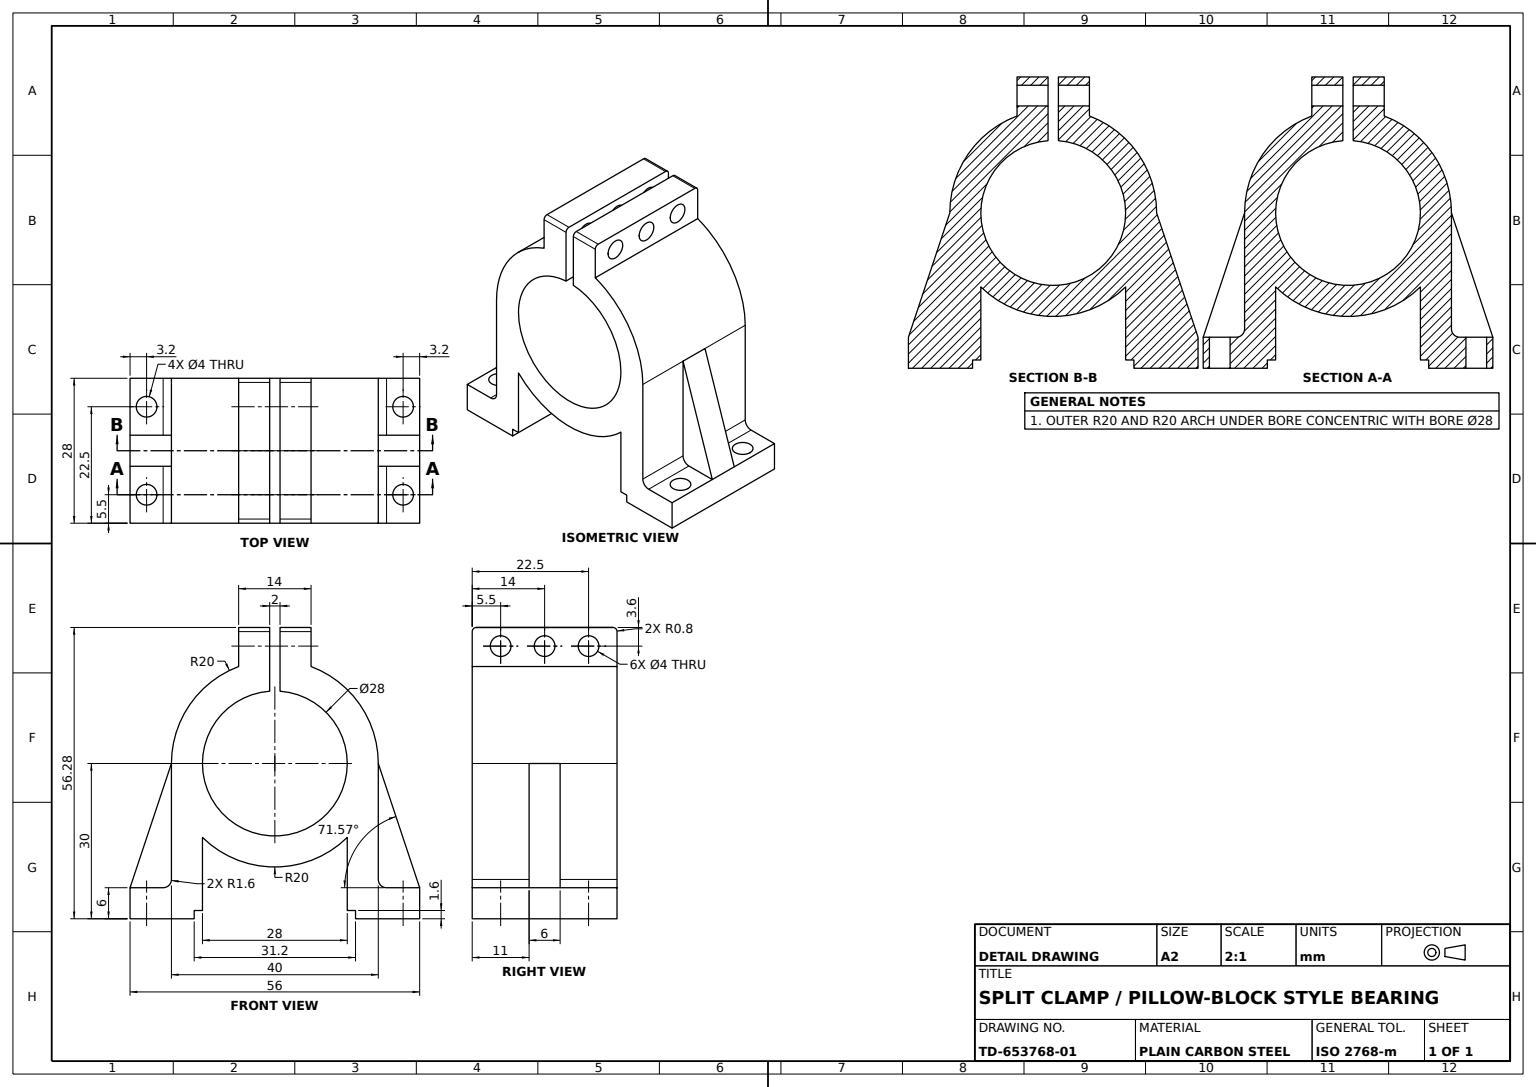
SolidWorks part; units mm, degrees
material "Plain Carbon Steel"
ref_plane "Front Plane" through (0, 0, 0) normal (0, 0, 1) x (1, 0, 0)
ref_plane "Top Plane" through (0, 0, 0) normal (0, 1, 0) x (1, 0, 0)
ref_plane "Right Plane" through (0, 0, 0) normal (1, 0, 0) x (0, 0, -1)
sketch "Clamp Body Profile" plane through (0, 0, 0) normal (0, 0, 1) x (1, 0, 0)
  line L6 (0, 0) -> (0, 4)
  line L7 (20, 24) -> (20, 0)
  line L8 (20, 0) -> (28, 0)
  line L9 (28, 0) -> (28, -6)
  line L16 (28, -6) -> (15.6, -6)
  line L17 (15.6, -6) -> (15.6, -4.4)
  line L18 (15.6, -4.4) -> (14, -4.4)
  line L19 (14, -4.4) -> (14, 9.7171)
  line L20 (-20, 24) -> (-20, 0)
  line L21 (-20, 0) -> (-28, 0)
  line L22 (-28, 0) -> (-28, -6)
  line L23 (-28, -6) -> (-15.6, -6)
  line L24 (-15.6, -6) -> (-15.6, -4.4)
  line L25 (-15.6, -4.4) -> (-14, -4.4)
  line L26 (-14, -4.4) -> (-14, 9.7171)
  arc A1 (-14, 9.7171) -> (14, 9.7171) centre (0, 24) ccw
  arc A2 (20, 24) -> (-20, 24) centre (0, 24) ccw
  dimension "D1" = 14
  dimension "D3" = 40
  dimension "D4" = 24
  dimension "D13" = 24
  dimension "D2" = 14
  dimension "D5" = 28
  dimension "D6" = 6
  dimension "D7" = 1.6
  dimension "D8" = 1.6
  dimension "D9" = 14.1171
  dimension "D10" = 6
  dimension "D11" = 1.6
  dimension "D12" = 6
extrude "Clamp Body" add sketch "Clamp Body Profile" along normal mid plane 28 contours L7 A2 L20 L21 L22 L23 L24 L25 L26 A1 L19 L18 L17 L16 L9 L8
sketch "Clamp Bore Sketch" plane through (0, 0, 14) normal (0, 0, 1) x (1, 0, 0)
  circle A0 centre (0, 24) radius 14
  dimension "D1" = 28
extrude "Clamp Bore" cut sketch "Clamp Bore Sketch" against normal blind 96
sketch "Clamp Lugs Sketch" plane through (0, 0, 14) normal (0, 0, 1) x (1, 0, 0)
  line L0 (0, 38) -> (7, 38)
  line L1 (7, 38) -> (7, 42.735)
  line L2 (7, 42.735) -> (7, 50.2788)
  line L3 (7, 50.2788) -> (-7, 50.2788)
  line L4 (-7, 50.2788) -> (-7, 38)
  line L5 (-7, 38) -> (0, 38)
  line L6 (-28, 0) -> (-28, -6) construction
  line L7 (-28, -6) -> (-15.6, -6) construction
  circle A0 centre (0, 24) radius 14 construction
  arc A1 (20, 24) -> (-20, 24) centre (0, 24) ccw construction
  dimension "D1" = 21
  dimension "D2" = 28
  dimension "D3" = 56.2788
extrude "Clamp Lugs" add sketch "Clamp Lugs Sketch" against normal blind 28
sketch "Split Slot Sketch" plane through (0, 0, 14) normal (0, 0, 1) x (1, 0, 0)
  line L0 (-1, 37.9642) -> (-1, 37.4063)
  line L1 (1, 38) -> (1, 50.2788)
  line L2 (7, 50.2788) -> (-7, 50.2788) construction
  line L3 (1, 50.2788) -> (-1, 50.2788)
  line L4 (-1, 50.2788) -> (-1, 37.9642)
  line L5 (-1, 37.4063) -> (1, 37.4063)
  line L6 (1, 37.4063) -> (1, 38)
  circle A0 centre (0, 24) radius 14 construction
  dimension "D1" = 2
  dimension "D2" = 12.2788
  dimension "D3" = 12.3145
  dimension "D4" = 12.8725
extrude "Split Slot 2mm" cut sketch "Split Slot Sketch" against normal blind 52
fillet "Body Fillet R1.6 A" radius 1.6 1 edges at (20, 0, 0)
fillet "Body Fillet R1.6 B" radius 1.6 1 edges at (-20, 0, 0)
sketch "Clamp Screw Holes Sketch" plane through (7, 0, 0) normal (1, 0, 0) x (0, 0, -1)
  line L0 (14, 42.735) -> (14, 50.2788) construction
  line L1 (14, 42.735) -> (-14, 42.735) construction
  circle A0 centre (8.5, 46.6788) radius 2
  circle A1 centre (-8.5, 46.6788) radius 2
  circle A2 centre (0, 46.6788) radius 2
  dimension "D1" = 4
  dimension "D2" = 5.5
  dimension "D3" = 14
  dimension "D4" = 22.5
  dimension "D5" = 3.9438
extrude "Clamp Screw Holes 3x" cut sketch "Clamp Screw Holes Sketch" against normal blind 52
sketch "Support Rib 1 Sketch" plane through (0, 0, 0) normal (0, 0, 1) x (1, 0, 0)
  line L0 (28, 0) -> (20, 24)
rib "Support Rib 1" sketch "Support Rib 1 Sketch" sketch "Support Rib 1 Sketch" thickness 6 extrusion direction parallel to sketch draft on no parameters "D1"=6
sketch "Support Rib 2 Sketch" plane through (0, 0, 0) normal (0, 0, 1) x (1, 0, 0)
  line L0 (-20, 24) -> (-28, 0)
rib "Support Rib 2" sketch "Support Rib 2 Sketch" sketch "Support Rib 2 Sketch" thickness 6 extrusion direction parallel to sketch draft on no parameters "D1"=6
sketch "Base Mounting Holes Sketch" plane through (0, 0, 0) normal (0, 1, 0) x (1, 0, 0)
  line L0 (21.6, -3) -> (21.6, -14) construction
  line L1 (21.6, -3) -> (28, -3) construction
  circle A0 centre (24.8, 8.5) radius 2
  circle A1 centre (24.8, -8.5) radius 2
  circle A2 centre (-24.8, 8.5) radius 2
  circle A3 centre (-24.8, -8.5) radius 2
  dimension "D1" = 4
  dimension "D2" = 3.2
  dimension "D3" = 46.4
  dimension "D4" = 11.5
  dimension "D5" = 5.5
extrude "Base Mounting Holes 4x" cut sketch "Base Mounting Holes Sketch" against normal blind 52
fillet "Lug Fillet R0.8 A" radius 0.8 1 edges at (4, 50.2788, 14)
fillet "Lug Fillet R0.8 B" radius 0.8 1 edges at (-4, 50.2788, 14)
fillet "Lug Fillet R0.8 C" radius 0.8 1 edges at (-4, 50.2788, -14)
fillet "Lug Fillet R0.8 D" radius 0.8 1 edges at (4, 50.2788, -14)
